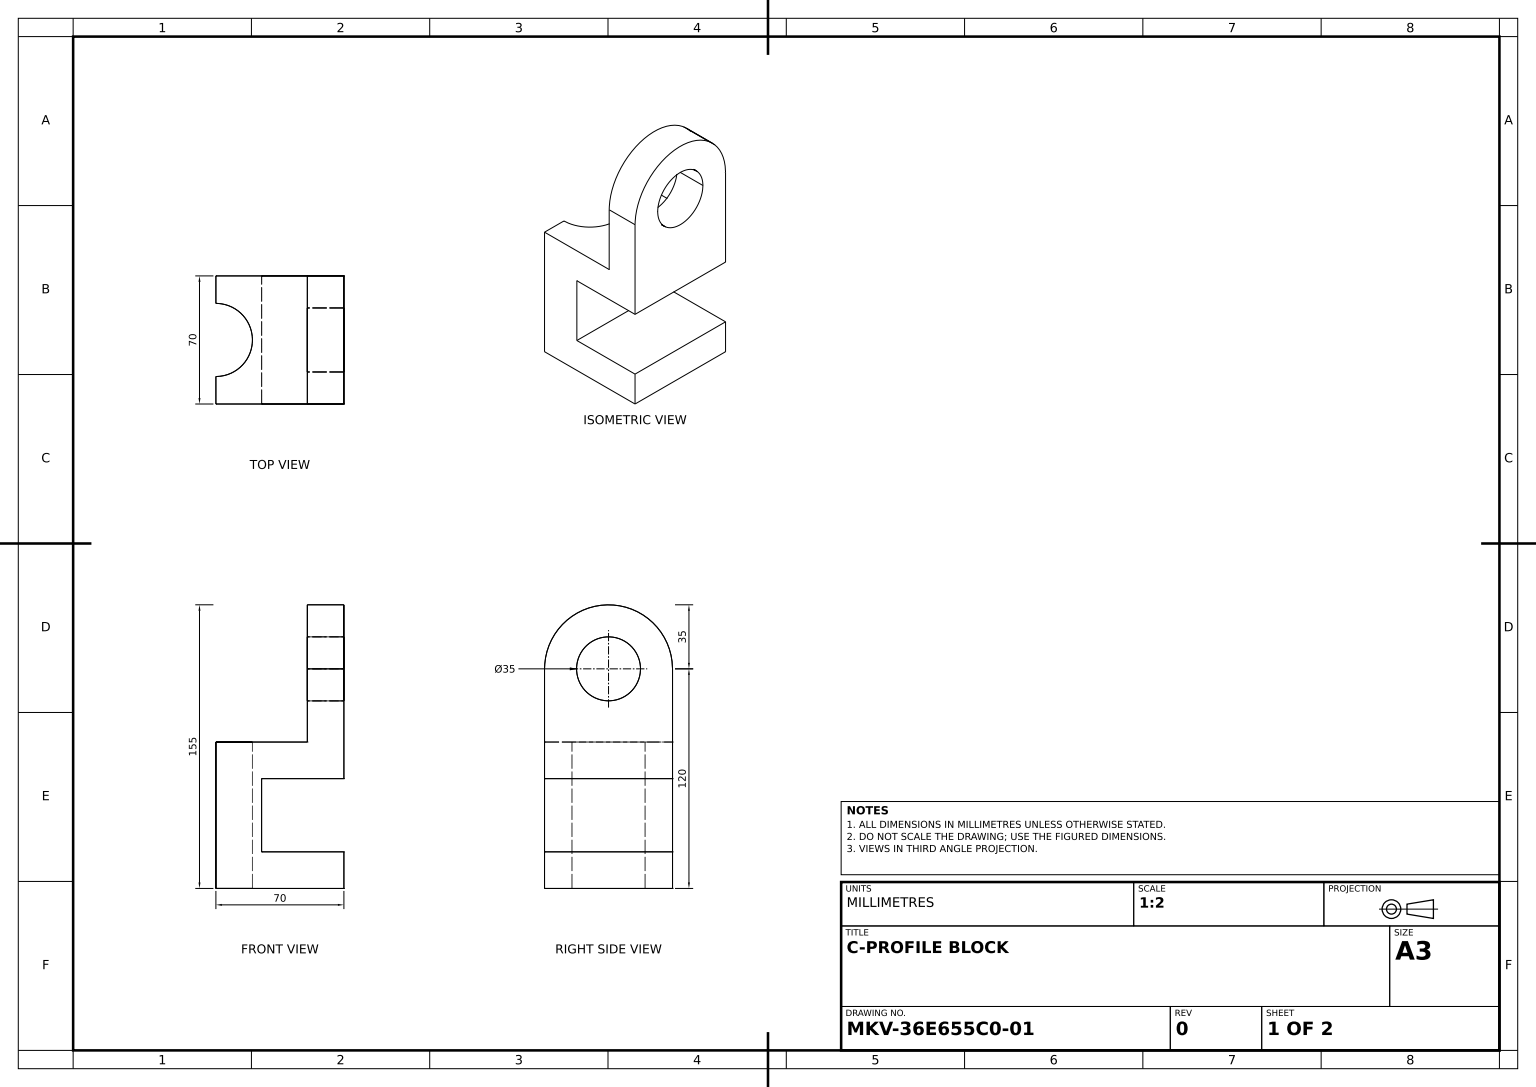
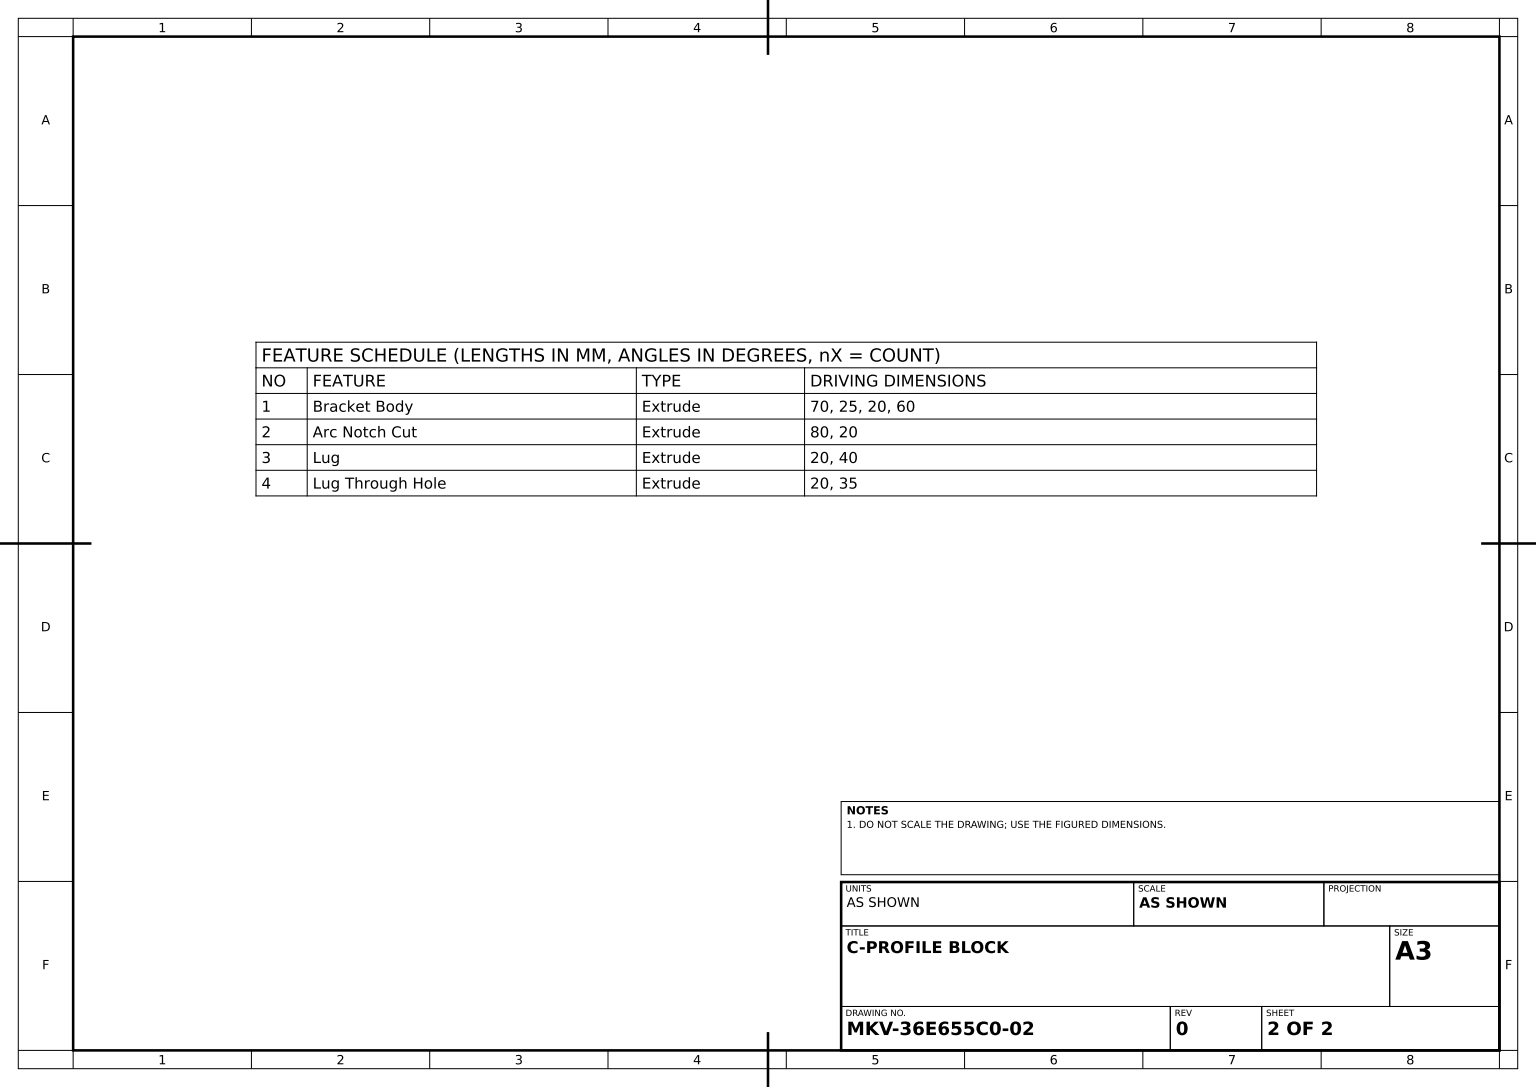
from build123d import *

# Parameters (mm, degrees)
BRACKET_BODY_DEPTH     = 70
ARC_NOTCH_CUT_DEPTH    = 80
LUG_DEPTH              = 20
LUG_HOLE_SKETCH_R      = 17.5
LUG_THROUGH_HOLE_DEPTH = 20


with BuildPart() as part:
    # Bracket Profile Sketch → Bracket Body (new body)
    with BuildSketch(Plane.XY):
        Polygon((0, 0), (70, 0), (70, 20), (25, 20), (25, 60), (70, 60), (70, 80), (0, 80), align=None)
    extrude(amount=BRACKET_BODY_DEPTH)

    # Arc Notch Sketch → Arc Notch Cut (cut)
    with BuildSketch(Plane(origin=(0, 80, 0), x_dir=(1, 0, 0), z_dir=(0, 1, 0))):
        with BuildLine():
            Line((0, -15), (0, -55))
            ThreePointArc((0, -55), (20, -35), (0, -15))
        make_face()
    extrude(amount=-ARC_NOTCH_CUT_DEPTH, mode=Mode.SUBTRACT)

    # Lug Profile Sketch → Lug (add)
    with BuildSketch(Plane(origin=(70, 0, 0), x_dir=(0, 0, -1), z_dir=(1, 0, 0))):
        with BuildLine():
            Line((-70, 120), (-70, 80))
            Line((-70, 80), (0, 80))
            Line((0, 80), (0, 120))
            ThreePointArc((0, 120), (-35, 155), (-70, 120))
        make_face()
    extrude(amount=-LUG_DEPTH)

    # Lug Hole Sketch → Lug Through Hole (cut)
    with BuildSketch(Plane.ZY.offset(-50)):
        with Locations((35, 120)):
            Circle(LUG_HOLE_SKETCH_R)
    extrude(amount=-LUG_THROUGH_HOLE_DEPTH, mode=Mode.SUBTRACT)


solid = part.part
